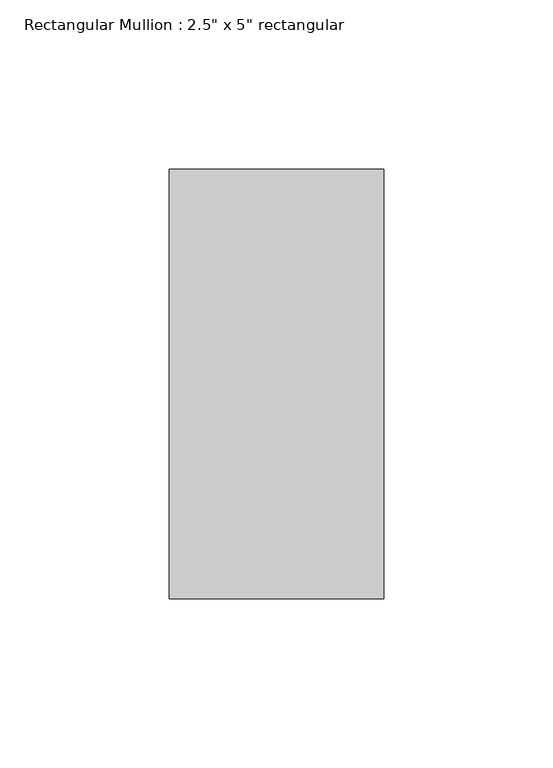
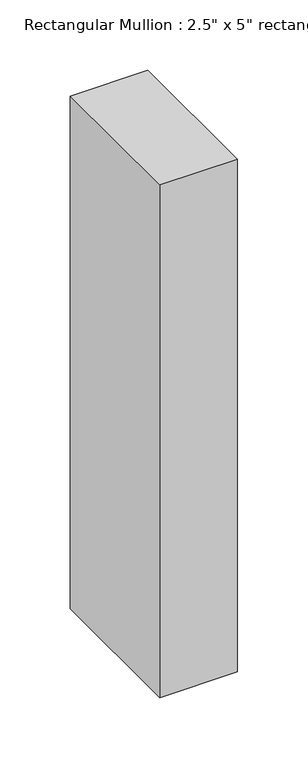
"""IFC4 building model written with IfcOpenShell, lengths in millimetres: member geometry."""

from ifc_helpers import new_model, si_unit, frame, origin, place, context, project, spatial, polyline, outline, extrude, source, transform, mapped, element, save


def member_bc7dbe04(model_context):
    return source(origin(), model_context, "Body", "SweptSolid", [
        extrude(outline(polyline([(0.0, 63.5), (0.0, -63.5), (-63.5, -63.5), (-63.5, 63.5), (0.0, 63.5)])), frame((0.0, 0.0, -444.5), z_axis=(0.0, 0.0, 1.0), x_axis=(1.0, 0.0, 0.0)), (0.0, 0.0, 1.0), 444.5),
    ])


if __name__ == "__main__":
    model = new_model("IFC4")
    model_context = context("Model", 3, world=origin())
    ifc_project = project(units=[si_unit("LENGTHUNIT", "METRE", prefix="MILLI")], contexts=[model_context])
    site = spatial("IfcSite", under=ifc_project)
    building = spatial("IfcBuilding", under=site)
    placement = place(None, origin())
    member_shape = member_bc7dbe04(model_context)
    element("IfcMember", 1, ObjectType="Rectangular Mullion : 2.5\" x 5\" rectangular", at=placement, inside=building, context=model_context, shape_type="MappedRepresentation", body=[
        mapped(member_shape, transform((0.0, 0.0, 0.0), x_axis=(1.0, 0.0, 0.0), y_axis=(0.0, 1.0, 0.0), z_axis=(0.0, 0.0, 1.0))),
    ])
    save(model, "model.ifc")

# Revit data of these elements
# Type "Rectangular Mullion : 2.5\" x 5\" rectangular"
#   built-in parameter 1007304 = 0.416667 (stored number, unit not read)
#   built-in parameter 1007301 = 0.104167 (stored number, unit not read)
#   built-in parameter 1007300 = 0.104167 (stored number, unit not read)
# Element 1 (IfcMember, "Rectangular Mullion : 2.5\" x 5\" rectangular")
#   Materials on its faces: "Aluminum"
# Materials
#   "Aluminum": class "Metal", colour RGB 247 247 247, transparency 0, Description = "Aluminum 6061", Cost = 0
